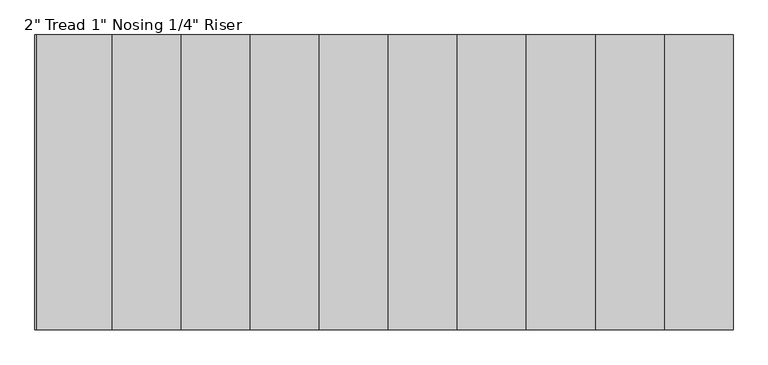
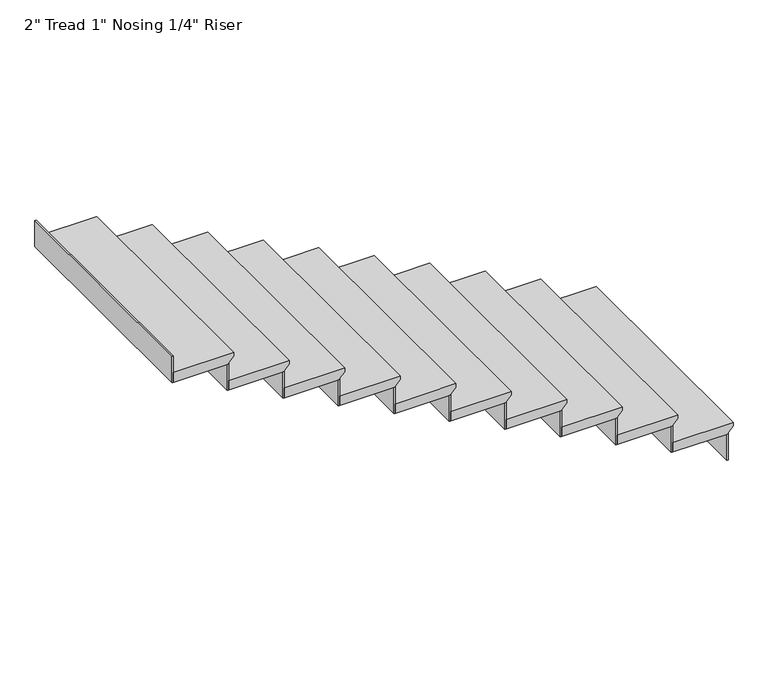
"""IFC4 building model written with IfcOpenShell, lengths in millimetres: stair flight geometry."""

from ifc_helpers import new_model, si_unit, frame, origin, place, context, project, spatial, polyline, outline, extrude, source, transform, mapped, element, save


def stair_flight_799f9057(model_context):
    return source(origin(), model_context, "Body", "SweptSolid", [
        extrude(outline(polyline([(1808.9217391, -9863.4532683), (1808.9217391, -10168.2532683), (1758.1217391, -10168.2532683), (1758.1217391, -9888.8532683), (1764.4717391, -9888.8532683), (1789.8717391, -9863.4532683), (1808.9217391, -9863.4532683)])), frame((0.0, 847.2393562, 0.0), z_axis=(0.0, 1.0, 0.0), x_axis=(0.0, 0.0, 1.0)), (0.0, 0.0, 1.0), 1193.8),
        extrude(outline(polyline([(-9895.2032683, 2041.0393562), (-9888.8532683, 2041.0393562), (-9888.8532683, 847.2393562), (-9895.2032683, 847.2393562), (-9895.2032683, 2041.0393562)])), frame((0.0, 0.0, 1618.973913), z_axis=(0.0, 0.0, 1.0), x_axis=(1.0, 0.0, 0.0)), (0.0, 0.0, 1.0), 139.1478261),
        extrude(outline(polyline([(-10174.6032683, 2041.0393562), (-10168.2532683, 2041.0393562), (-10168.2532683, 847.2393562), (-10174.6032683, 847.2393562), (-10174.6032683, 2041.0393562)])), frame((0.0, 0.0, 1758.1217391), z_axis=(0.0, 0.0, 1.0), x_axis=(1.0, 0.0, 0.0)), (0.0, 0.0, 1.0), 139.1478261),
        extrude(outline(polyline([(1948.0695652, -10142.8532683), (1948.0695652, -10447.6532683), (1897.2695652, -10447.6532683), (1897.2695652, -10168.2532683), (1903.6195652, -10168.2532683), (1929.0195652, -10142.8532683), (1948.0695652, -10142.8532683)])), frame((0.0, 847.2393562, 0.0), z_axis=(0.0, 1.0, 0.0), x_axis=(0.0, 0.0, 1.0)), (0.0, 0.0, 1.0), 1193.8),
        extrude(outline(polyline([(-10454.0032683, 2041.0393562), (-10447.6532683, 2041.0393562), (-10447.6532683, 847.2393562), (-10454.0032683, 847.2393562), (-10454.0032683, 2041.0393562)])), frame((0.0, 0.0, 1897.2695652), z_axis=(0.0, 0.0, 1.0), x_axis=(1.0, 0.0, 0.0)), (0.0, 0.0, 1.0), 139.1478261),
        extrude(outline(polyline([(2087.2173913, -10422.2532683), (2087.2173913, -10727.0532683), (2036.4173913, -10727.0532683), (2036.4173913, -10447.6532683), (2042.7673913, -10447.6532683), (2068.1673913, -10422.2532683), (2087.2173913, -10422.2532683)])), frame((0.0, 847.2393562, 0.0), z_axis=(0.0, 1.0, 0.0), x_axis=(0.0, 0.0, 1.0)), (0.0, 0.0, 1.0), 1193.8),
        extrude(outline(polyline([(-10733.4032683, 2041.0393562), (-10727.0532683, 2041.0393562), (-10727.0532683, 847.2393562), (-10733.4032683, 847.2393562), (-10733.4032683, 2041.0393562)])), frame((0.0, 0.0, 2036.4173913), z_axis=(0.0, 0.0, 1.0), x_axis=(1.0, 0.0, 0.0)), (0.0, 0.0, 1.0), 139.1478261),
        extrude(outline(polyline([(2226.3652174, -10701.6532683), (2226.3652174, -11006.4532683), (2175.5652174, -11006.4532683), (2175.5652174, -10727.0532683), (2181.9152174, -10727.0532683), (2207.3152174, -10701.6532683), (2226.3652174, -10701.6532683)])), frame((0.0, 847.2393562, 0.0), z_axis=(0.0, 1.0, 0.0), x_axis=(0.0, 0.0, 1.0)), (0.0, 0.0, 1.0), 1193.8),
        extrude(outline(polyline([(-11012.8032683, 2041.0393562), (-11006.4532683, 2041.0393562), (-11006.4532683, 847.2393562), (-11012.8032683, 847.2393562), (-11012.8032683, 2041.0393562)])), frame((0.0, 0.0, 2175.5652174), z_axis=(0.0, 0.0, 1.0), x_axis=(1.0, 0.0, 0.0)), (0.0, 0.0, 1.0), 139.1478261),
        extrude(outline(polyline([(2365.5130435, -10981.0532683), (2365.5130435, -11285.8532683), (2314.7130435, -11285.8532683), (2314.7130435, -11006.4532683), (2321.0630435, -11006.4532683), (2346.4630435, -10981.0532683), (2365.5130435, -10981.0532683)])), frame((0.0, 847.2393562, 0.0), z_axis=(0.0, 1.0, 0.0), x_axis=(0.0, 0.0, 1.0)), (0.0, 0.0, 1.0), 1193.8),
        extrude(outline(polyline([(-11292.2032683, 2041.0393562), (-11285.8532683, 2041.0393562), (-11285.8532683, 847.2393562), (-11292.2032683, 847.2393562), (-11292.2032683, 2041.0393562)])), frame((0.0, 0.0, 2314.7130435), z_axis=(0.0, 0.0, 1.0), x_axis=(1.0, 0.0, 0.0)), (0.0, 0.0, 1.0), 139.1478261),
        extrude(outline(polyline([(2504.6608696, -11260.4532683), (2504.6608696, -11565.2532683), (2453.8608696, -11565.2532683), (2453.8608696, -11285.8532683), (2460.2108696, -11285.8532683), (2485.6108696, -11260.4532683), (2504.6608696, -11260.4532683)])), frame((0.0, 847.2393562, 0.0), z_axis=(0.0, 1.0, 0.0), x_axis=(0.0, 0.0, 1.0)), (0.0, 0.0, 1.0), 1193.8),
        extrude(outline(polyline([(-11571.6032683, 2041.0393562), (-11565.2532683, 2041.0393562), (-11565.2532683, 847.2393562), (-11571.6032683, 847.2393562), (-11571.6032683, 2041.0393562)])), frame((0.0, 0.0, 2453.8608696), z_axis=(0.0, 0.0, 1.0), x_axis=(1.0, 0.0, 0.0)), (0.0, 0.0, 1.0), 139.1478261),
        extrude(outline(polyline([(2643.8086957, -11539.8532683), (2643.8086957, -11844.6532683), (2593.0086957, -11844.6532683), (2593.0086957, -11565.2532683), (2599.3586957, -11565.2532683), (2624.7586957, -11539.8532683), (2643.8086957, -11539.8532683)])), frame((0.0, 847.2393562, 0.0), z_axis=(0.0, 1.0, 0.0), x_axis=(0.0, 0.0, 1.0)), (0.0, 0.0, 1.0), 1193.8),
        extrude(outline(polyline([(-11851.0032683, 2041.0393562), (-11844.6532683, 2041.0393562), (-11844.6532683, 847.2393562), (-11851.0032683, 847.2393562), (-11851.0032683, 2041.0393562)])), frame((0.0, 0.0, 2593.0086957), z_axis=(0.0, 0.0, 1.0), x_axis=(1.0, 0.0, 0.0)), (0.0, 0.0, 1.0), 139.1478261),
        extrude(outline(polyline([(2782.9565217, -11819.2532683), (2782.9565217, -12124.0532683), (2732.1565217, -12124.0532683), (2732.1565217, -11844.6532683), (2738.5065217, -11844.6532683), (2763.9065217, -11819.2532683), (2782.9565217, -11819.2532683)])), frame((0.0, 847.2393562, 0.0), z_axis=(0.0, 1.0, 0.0), x_axis=(0.0, 0.0, 1.0)), (0.0, 0.0, 1.0), 1193.8),
        extrude(outline(polyline([(-12130.4032683, 2041.0393562), (-12124.0532683, 2041.0393562), (-12124.0532683, 847.2393562), (-12130.4032683, 847.2393562), (-12130.4032683, 2041.0393562)])), frame((0.0, 0.0, 2732.1565217), z_axis=(0.0, 0.0, 1.0), x_axis=(1.0, 0.0, 0.0)), (0.0, 0.0, 1.0), 139.1478261),
        extrude(outline(polyline([(2922.1043478, -12098.6532683), (2922.1043478, -12403.4532683), (2871.3043478, -12403.4532683), (2871.3043478, -12124.0532683), (2877.6543478, -12124.0532683), (2903.0543478, -12098.6532683), (2922.1043478, -12098.6532683)])), frame((0.0, 847.2393562, 0.0), z_axis=(0.0, 1.0, 0.0), x_axis=(0.0, 0.0, 1.0)), (0.0, 0.0, 1.0), 1193.8),
        extrude(outline(polyline([(-12409.8032683, 2041.0393562), (-12403.4532683, 2041.0393562), (-12403.4532683, 847.2393562), (-12409.8032683, 847.2393562), (-12409.8032683, 2041.0393562)])), frame((0.0, 0.0, 2871.3043478), z_axis=(0.0, 0.0, 1.0), x_axis=(1.0, 0.0, 0.0)), (0.0, 0.0, 1.0), 139.1478261),
        extrude(outline(polyline([(-12689.2032683, 2041.0393562), (-12682.8532683, 2041.0393562), (-12682.8532683, 847.2393562), (-12689.2032683, 847.2393562), (-12689.2032683, 2041.0393562)])), frame((0.0, 0.0, 3010.4521739), z_axis=(0.0, 0.0, 1.0), x_axis=(1.0, 0.0, 0.0)), (0.0, 0.0, 1.0), 139.1478261),
        extrude(outline(polyline([(3061.2521739, -12378.0532683), (3061.2521739, -12682.8532683), (3010.4521739, -12682.8532683), (3010.4521739, -12403.4532683), (3016.8021739, -12403.4532683), (3042.2021739, -12378.0532683), (3061.2521739, -12378.0532683)])), frame((0.0, 847.2393562, 0.0), z_axis=(0.0, 1.0, 0.0), x_axis=(0.0, 0.0, 1.0)), (0.0, 0.0, 1.0), 1193.8),
    ])


if __name__ == "__main__":
    model = new_model("IFC4")
    model_context = context("Model", 3, world=origin())
    ifc_project = project(units=[si_unit("LENGTHUNIT", "METRE", prefix="MILLI")], contexts=[model_context])
    site = spatial("IfcSite", under=ifc_project)
    building = spatial("IfcBuilding", under=site)
    placement = place(None, origin())
    stair_flight_shape = stair_flight_799f9057(model_context)
    element("IfcStairFlight", 1, ObjectType="2\" Tread 1\" Nosing 1/4\" Riser", at=placement, inside=building, context=model_context, shape_type="MappedRepresentation", body=[
        mapped(stair_flight_shape, transform((0.0, 0.0, 0.0), x_axis=(1.0, 0.0, 0.0), y_axis=(0.0, 1.0, 0.0), z_axis=(0.0, 0.0, 1.0))),
    ])
    save(model, "model.ifc")
